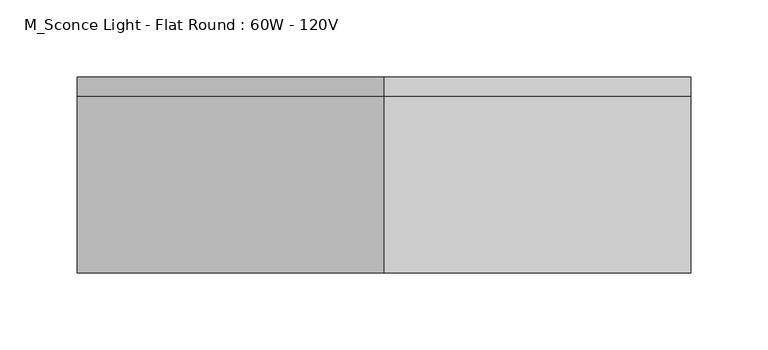
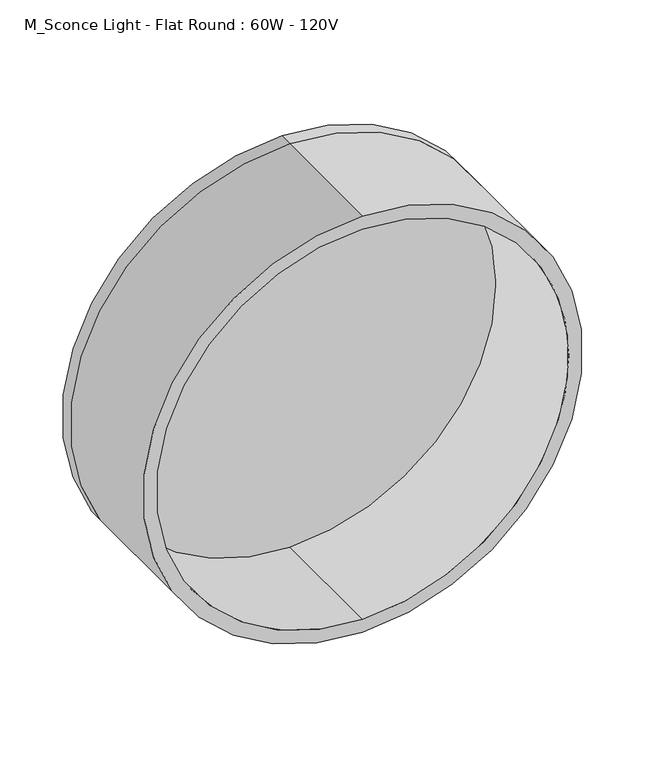
"""IFC4 building model written with IfcOpenShell, lengths in millimetres: light fixture geometry, M_Sconce Light - Flat Round : 60W - 120V."""

from ifc_helpers import new_model, si_unit, point, frame, frame_2d, origin, place, context, project, spatial, circle_curve, trimmed, segment, composite_curve, outline, extrude, source, transform, mapped, element, save


def m_sconce_light_flat_round_60w_120v_dc625014(model_context):
    return source(origin(), model_context, "Body", "SweptSolid", [
        extrude(outline(composite_curve([segment(trimmed(circle_curve(frame_2d((1900.0, 0.0)), 200.0), [point((1700.0, 0.0))], [point((2100.0, 0.0))], False, "CARTESIAN"), True, "CONTINUOUS"), segment(trimmed(circle_curve(frame_2d((1900.0, 0.0)), 200.0), [point((2100.0, 0.0))], [point((1700.0, 0.0))], False, "CARTESIAN"), True, "CONTINUOUS")], self_intersect=False), holes=[composite_curve([segment(trimmed(circle_curve(frame_2d((1900.0, 0.0)), 187.5182302), [point((1712.4817698, 0.0))], [point((2087.5182302, 0.0))], True, "CARTESIAN"), True, "CONTINUOUS"), segment(trimmed(circle_curve(frame_2d((1900.0, 0.0)), 187.5182302), [point((2087.5182302, 0.0))], [point((1712.4817698, 0.0))], True, "CARTESIAN"), True, "CONTINUOUS")], self_intersect=False)]), frame((0.0, 114.3, 0.0), z_axis=(0.0, 1.0, 0.0), x_axis=(0.0, 0.0, 1.0)), (0.0, 0.0, 1.0), 114.3),
        extrude(outline(composite_curve([segment(trimmed(circle_curve(frame_2d((1900.0, 0.0)), 200.0), [point((1700.0, 0.0))], [point((2100.0, 0.0))], False, "CARTESIAN"), True, "CONTINUOUS"), segment(trimmed(circle_curve(frame_2d((1900.0, 0.0)), 200.0), [point((2100.0, 0.0))], [point((1700.0, 0.0))], False, "CARTESIAN"), True, "CONTINUOUS")], self_intersect=False)), frame((0.0, 228.6, 0.0), z_axis=(0.0, 1.0, 0.0), x_axis=(0.0, 0.0, 1.0)), (0.0, 0.0, 1.0), 12.7),
    ])


if __name__ == "__main__":
    model = new_model("IFC4")
    model_context = context("Model", 3, world=origin())
    ifc_project = project(units=[si_unit("LENGTHUNIT", "METRE", prefix="MILLI")], contexts=[model_context])
    site = spatial("IfcSite", under=ifc_project)
    building = spatial("IfcBuilding", under=site)
    placement = place(None, origin())
    m_sconce_light_flat_round_60w_120v_shape = m_sconce_light_flat_round_60w_120v_dc625014(model_context)
    element("IfcLightFixture", 1, ObjectType="M_Sconce Light - Flat Round : 60W - 120V", at=placement, inside=building, context=model_context, shape_type="MappedRepresentation", body=[
        mapped(m_sconce_light_flat_round_60w_120v_shape, transform((0.0, 0.0, 0.0), x_axis=(1.0, 0.0, 0.0), y_axis=(0.0, 1.0, 0.0), z_axis=(0.0, 0.0, 1.0))),
    ])
    save(model, "model.ifc")

# Revit data of these elements
# Type "M_Sconce Light - Flat Round : 60W - 120V"
#   Assembly Code = "D5020220"
#   Lamp = "A-19"
#   Wattage = 60 W
#   built-in parameter 1150110 = 1 (stored number, unit not read)
#   built-in parameter 1114217 = 1 (stored number, unit not read)
#   built-in parameter 1150109 = 1 (stored number, unit not read)
#   built-in parameter 1150113 = 1 (stored number, unit not read)
#   built-in parameter 1150115 = 1 (stored number, unit not read)
#   built-in parameter 1150105 = 272.155 (stored number, unit not read)
#   Light Source Symbol Size = 2' - 0"
#   built-in parameter 1150112 = 1 (stored number, unit not read)
#   built-in parameter 1150114 = 1 (stored number, unit not read)
#   built-in parameter 1150107 = 2800 (stored number, unit not read)
#   built-in parameter 1150106 = 2.72155 (stored number, unit not read)
#   built-in parameter 1150104 = 1.32387 (stored number, unit not read)
#   Ballast Voltage = 120 V
#   built-in parameter 1114218 = 1 (stored number, unit not read)
#   built-in parameter 1150133 = 10 (stored number, unit not read)
#   Lumens = 855 lm
#   Mounting Height = 6' - 2.80315"
#   Radius = 0' - 7.87402"
#   Apparent Load = 60 VA
#   built-in parameter 1150134 = 4
#   built-in parameter 1150137 = 1
#   Color Filter = 16777215
#   built-in parameter 1140040 [instance default] = 1
#   Ballast Number of Poles = 1
#   Shade Material = Glass, Frosted
#   Dimming Lamp Color Temperature Shift = (empty or 0)
#   Default Elevation = 0
#   Wattage Comments = ""
# Element 1 (IfcLightFixture, "M_Sconce Light - Flat Round : 60W - 120V")
#   Materials on its faces: "Glass, Frosted"
# Materials
#   "Glass, Frosted": class "Glass", colour RGB 250 244 225, transparency 0.55, Description = "physical material", Cost = 0
